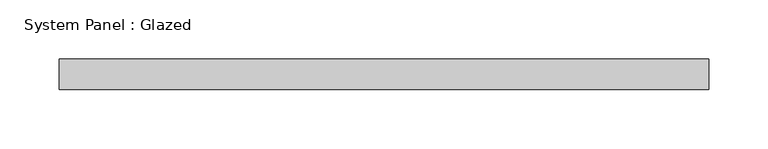
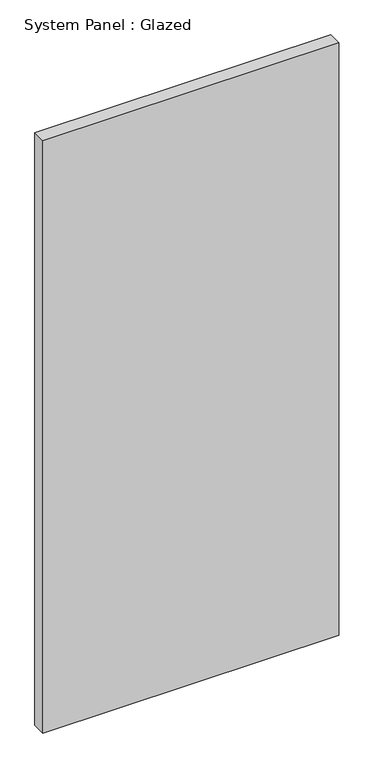
"""IFC4 building model written with IfcOpenShell, lengths in millimetres: plate geometry, System Panel : Glazed."""

from ifc_helpers import new_model, si_unit, origin, origin_with_axes, place, context, project, spatial, polyline, outline, extrude, source, transform, mapped, element, save


def system_panel_glazed_8be6732c(model_context):
    return source(origin(), model_context, "Body", "SweptSolid", [
        extrude(outline(polyline([(273.05, 19.05), (-273.05, 19.05), (-273.05, 44.45), (273.05, 44.45), (273.05, 19.05)])), origin_with_axes(), (0.0, 0.0, 1.0), 1155.7),
    ])


if __name__ == "__main__":
    model = new_model("IFC4")
    model_context = context("Model", 3, world=origin())
    ifc_project = project(units=[si_unit("LENGTHUNIT", "METRE", prefix="MILLI")], contexts=[model_context])
    site = spatial("IfcSite", under=ifc_project)
    building = spatial("IfcBuilding", under=site)
    placement = place(None, origin())
    system_panel_glazed_shape = system_panel_glazed_8be6732c(model_context)
    element("IfcPlate", 1, ObjectType="System Panel : Glazed", at=placement, inside=building, context=model_context, shape_type="MappedRepresentation", body=[
        mapped(system_panel_glazed_shape, transform((0.0, 0.0, 0.0), x_axis=(1.0, 0.0, 0.0), y_axis=(0.0, 1.0, 0.0), z_axis=(0.0, 0.0, 1.0))),
    ])
    save(model, "model.ifc")

# Revit data of these elements
# Type "System Panel : Glazed"
#   Construction Type Id = "GSP4R"
#   Analytic Construction = "1/8 in Pilkington single glazing"
#   Visual Light Transmittance = 0.9
#   Solar Heat Gain Coefficient = 0.86
#   Heat Transfer Coefficient (U) = 1.18115 BTU/(h·ft²·°F)
# Element 1 (IfcPlate, "System Panel : Glazed")
#   Materials on its faces: "Glass"
# Materials
#   "Glass": class "Glass", colour RGB 0 128 192, transparency 0.75, Description = "Soda Lime Glass", Cost = 0
